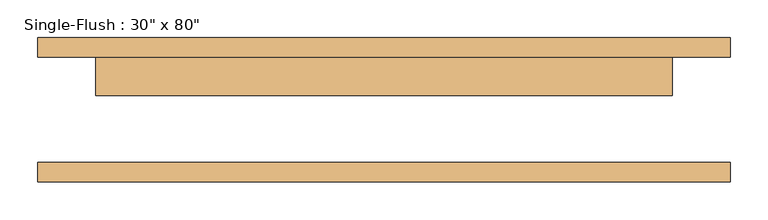
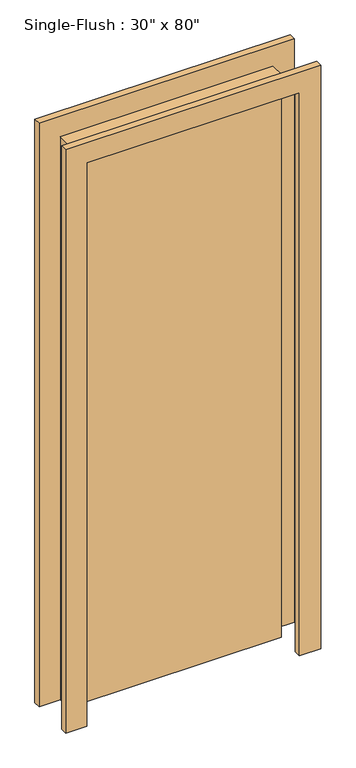
"""IFC4 building model written with IfcOpenShell, lengths in millimetres: door geometry."""

from ifc_helpers import new_model, si_unit, frame, origin, origin_with_axes, place, context, project, spatial, polyline, outline, extrude, source, transform, mapped, element, save


def door_6d488673(model_context):
    return source(origin(), model_context, "Body", "SweptSolid", [
        extrude(outline(polyline([(2209.8, -457.2), (0.0, -457.2), (0.0, -381.0), (2133.6, -381.0), (2133.6, 381.0), (0.0, 381.0), (0.0, 457.2), (2209.8, 457.2), (2209.8, -457.2)])), frame((0.0, 69.85, 0.0), z_axis=(0.0, 1.0, 0.0), x_axis=(0.0, 0.0, 1.0)), (0.0, 0.0, 1.0), 25.4),
        extrude(outline(polyline([(2209.8, 457.2), (2209.8, -457.2), (0.0, -457.2), (0.0, -381.0), (2133.6, -381.0), (2133.6, 381.0), (0.0, 381.0), (0.0, 457.2), (2209.8, 457.2)])), frame((0.0, -95.25, 0.0), z_axis=(0.0, 1.0, 0.0), x_axis=(0.0, 0.0, 1.0)), (0.0, 0.0, 1.0), 25.4),
        extrude(outline(polyline([(381.0, 19.05), (-381.0, 19.05), (-381.0, 69.85), (381.0, 69.85), (381.0, 19.05)])), origin_with_axes(), (0.0, 0.0, 1.0), 2133.6),
    ])


if __name__ == "__main__":
    model = new_model("IFC4")
    model_context = context("Model", 3, world=origin())
    ifc_project = project(units=[si_unit("LENGTHUNIT", "METRE", prefix="MILLI")], contexts=[model_context])
    site = spatial("IfcSite", under=ifc_project)
    building = spatial("IfcBuilding", under=site)
    placement = place(None, origin())
    door_shape = door_6d488673(model_context)
    element("IfcDoor", 1, ObjectType="Single-Flush : 30\" x 80\"", at=placement, inside=building, context=model_context, shape_type="MappedRepresentation", body=[
        mapped(door_shape, transform((0.0, 0.0, 0.0), x_axis=(1.0, 0.0, 0.0), y_axis=(0.0, 1.0, 0.0), z_axis=(0.0, 0.0, 1.0))),
    ])
    save(model, "model.ifc")

# Revit data of these elements
# Type "Single-Flush : 30\" x 80\""
#   Type Mark = "5"
#   Construction Type Id = "MDOOR"
#   Assembly Code = "C1020"
#   Analytic Construction = "Metal"
#   Thickness = 0' - 2"
#   Heat Transfer Coefficient (U) = 0.651978 BTU/(h·ft²·°F)
#   Height = 7' - 0"
#   Trim Projection Ext = 0' - 1"
#   Trim Projection Int = 0' - 1"
#   Trim Width = 0' - 3"
#   Width = 2' - 6"
#   Define Thermal Properties by = 1
#   Define Thermal Properties by = 1
#   Door Material = Door - Panel
#   Frame Material = Door - Frame
#   Visual Light Transmittance = 0
#   Solar Heat Gain Coefficient = 0
#   Function = (empty or 0)
#   Wall Closure = (empty or 0)
# Element 1 (IfcDoor, "Single-Flush : 30\" x 80\"")
#   Materials on its faces: "Door - Frame", "Door - Panel"
# Materials
#   "Door - Panel": class "Wood", colour RGB 210 159 95, transparency 0, Cost = 0
#   "Door - Frame": colour RGB 118 70 51, transparency 0, Cost = 0
